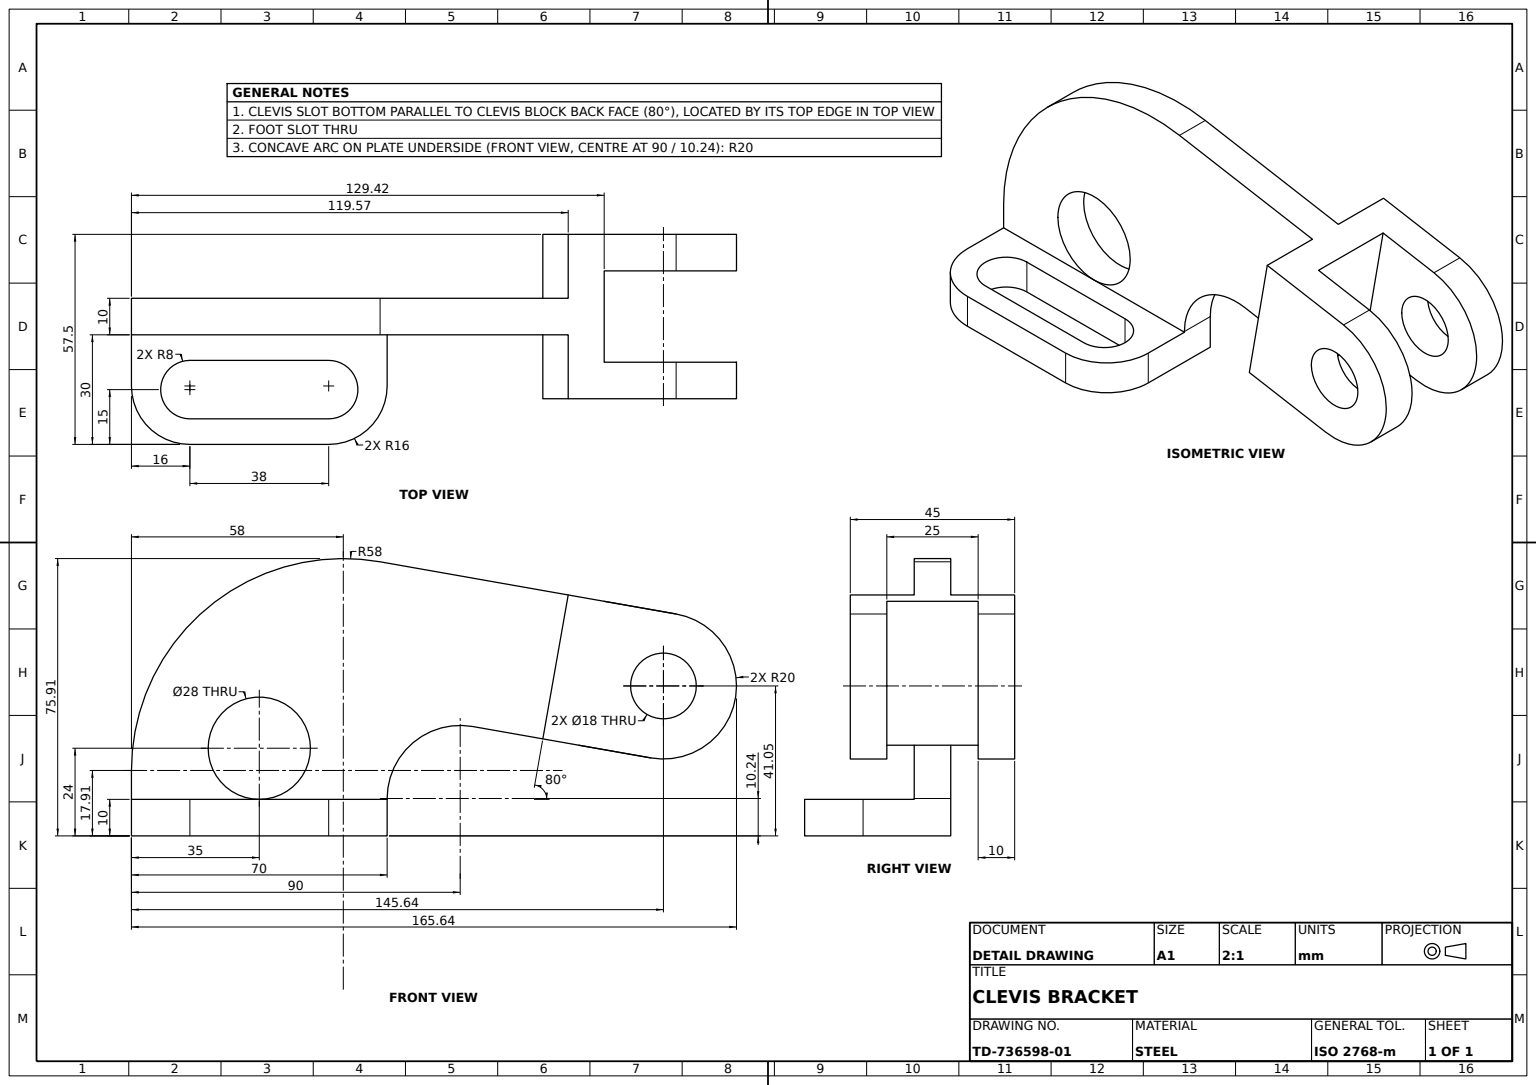
from build123d import *

# Parameters (mm, degrees)
ARCHED_PLATE_PROFILE_R      = 14
ARCHED_BASE_PLATE_DEPTH     = 5
SLOTTED_MOUNTING_FOOT_DEPTH = 10
CLEVIS_BLOCK_PROFILE_W      = 45
CLEVIS_BLOCK_PROFILE_H      = 40
CLEVIS_BLOCK_DEPTH          = 50
PLATE_EDGE_FILLET_RADIUS    = 20
PLATE_EDGE_FILLET_LENGTH    = 45
CLEVIS_PIN_HOLE_PROFILE_R   = 9
CLEVIS_PIN_HOLE_18_DEPTH    = 50
CLEVIS_SLOT_PROFILE_W       = 50
CLEVIS_SLOT_PROFILE_H       = 25
CLEVIS_SLOT_DEPTH           = 50


with BuildPart() as part:
    # Arched Plate Profile → Arched Base Plate (new, symmetric)
    with BuildSketch(Plane.XY):
        with BuildLine():
            Line((0, 0), (0, 17.91362622))
            ThreePointArc((0, 17.91362622), (20.718318638, 62.344203921), (68.071594305, 75.032475895))
            Line((68.071594305, 75.032475895), (119.569687178, 65.951972666))
            Line((119.569687178, 65.951972666), (112.623760072, 26.559662546))
            Line((112.623760072, 26.559662546), (93.472963553, 29.936464674))
            ThreePointArc((93.472963553, 29.936464674), (77.144247806, 25.561198476), (70, 10.240309613))
            Line((70, 10.240309613), (70, 0))
            Line((70, 0), (0, 0))
        make_face()
        with Locations((35, 24)):
            Circle(ARCHED_PLATE_PROFILE_R, mode=Mode.SUBTRACT)
    extrude(amount=ARCHED_BASE_PLATE_DEPTH, both=True)

    # Slotted Foot Profile → Slotted Mounting Foot (add)
    with BuildSketch(Plane(origin=(0, 0, 0), x_dir=(1, 0, 0), z_dir=(0, 1, 0))):
        with BuildLine():
            Line((0, -5), (70, -5))
            Line((70, -5), (70, -19))
            ThreePointArc((70, -19), (65.313708499, -30.313708499), (54, -35))
            Line((54, -35), (16, -35))
            ThreePointArc((16, -35), (4.686291501, -30.313708499), (0, -19))
            Line((0, -19), (0, -5))
        make_face()
        with BuildLine():
            Line((16, -12), (54, -12))
            ThreePointArc((54, -12), (62, -20), (54, -28))
            Line((54, -28), (16, -28))
            ThreePointArc((16, -28), (8, -20), (16, -12))
        make_face(mode=Mode.SUBTRACT)
    extrude(amount=SLOTTED_MOUNTING_FOOT_DEPTH)

    # Clevis Block Profile → Clevis Block (add)
    with BuildSketch(Plane(origin=(104.685768373, -18.45892546, 0), x_dir=(0, 0, -1), z_dir=(0.9848077530122075, -0.17364817766693413, 0))):
        with Locations((0, 65.713072291)):
            Rectangle(CLEVIS_BLOCK_PROFILE_W, CLEVIS_BLOCK_PROFILE_H)
    extrude(amount=CLEVIS_BLOCK_DEPTH)

    # Plate Edge Fillet: full round fillet: the end face becomes a half cylinder, R = half its width
    plate_edge_fillet_face = Plane((165.337111276, 37.573408722, 0), x_dir=(0, 0, -1), z_dir=(0.984807753012, -0.173648177667, 0))  # on the end face: x along it, z out of the body
    plate_edge_fillet_slab = plate_edge_fillet_face.offset(-PLATE_EDGE_FILLET_RADIUS / 2) * Box(PLATE_EDGE_FILLET_LENGTH, 2 * PLATE_EDGE_FILLET_RADIUS, PLATE_EDGE_FILLET_RADIUS, mode=Mode.PRIVATE)  # the body's end, R deep
    plate_edge_fillet_round = Plane((145.640956216, 41.046372275, 0), x_dir=(0.984807753012, -0.173648177667, 0), z_dir=(0, 0, -1)) * Cylinder(PLATE_EDGE_FILLET_RADIUS, PLATE_EDGE_FILLET_LENGTH, mode=Mode.PRIVATE)  # its axis R under the face
    add(plate_edge_fillet_slab - plate_edge_fillet_round, mode=Mode.SUBTRACT)

    # Clevis Pin Hole Profile → Clevis Pin Hole _18 (cut)
    with BuildSketch(Plane.XY.offset(22.5)):
        with Locations((145.640956215, 41.046372276)):
            Circle(CLEVIS_PIN_HOLE_PROFILE_R)
    extrude(amount=-CLEVIS_PIN_HOLE_18_DEPTH, mode=Mode.SUBTRACT)

    # Clevis Slot Profile → Clevis Slot (cut)
    with BuildSketch(Plane(origin=(14.883918806, 84.410898126, 0), x_dir=(0.9848077530122074, -0.17364817766693438, 0), z_dir=(0.17364817766693438, 0.9848077530122074, 0))):
        with Locations((141.300715091, 0)):
            Rectangle(CLEVIS_SLOT_PROFILE_W, CLEVIS_SLOT_PROFILE_H)
    extrude(amount=-CLEVIS_SLOT_DEPTH, mode=Mode.SUBTRACT)


solid = part.part
